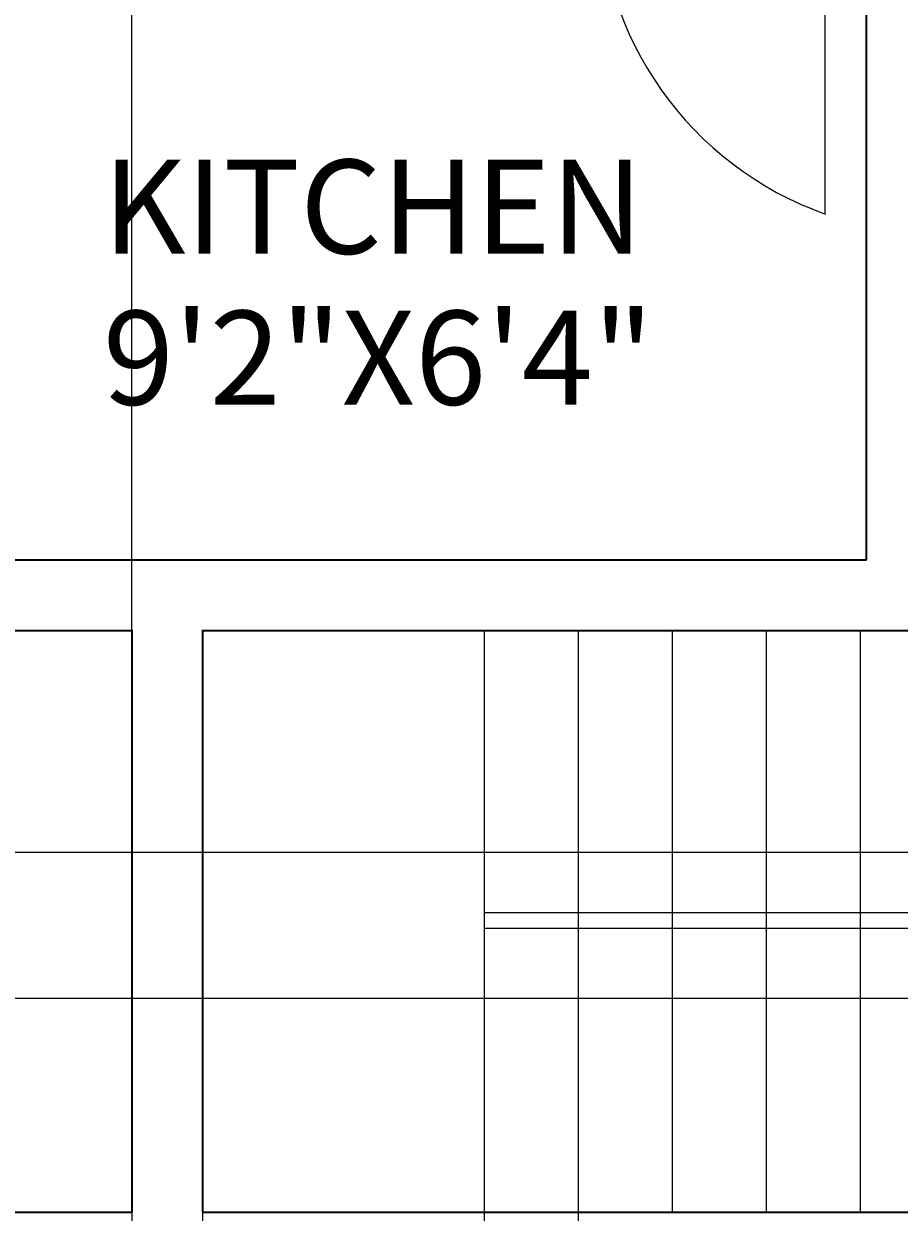
# Model space of a CAD drawing. Units: feet. Extents: x 5816 to 6644, y 25475 to 26788.
# Tile 4 of 23: x 5940 to 6052, y 26094 to 26246. Entities that reach past the tile are written whole.
import ezdxf

# ---------------------------------------------------------------- set-up
doc = ezdxf.new("R2010")
doc.units = ezdxf.units.FT
for name, color, linetype, lineweight in [('A-ANNO-DIMS', 2, 'Continuous', 13), ('A-AREA-IDEN', 7, 'Continuous', 18), ('A-DOOR', 3, 'Continuous', 18), ('A-FLOR-STRS', 7, 'Continuous', 18), ('A-WALL', 7, 'Continuous', 35)]:
    doc.layers.add(name, color=color, linetype=linetype, lineweight=lineweight)
doc.styles.get("Standard").update_dxf_attribs({"font": 'arial.ttf'})
doc.dimstyles.get("Standard").update_dxf_attribs({"dimtxt": 0.18, "dimasz": 0.18, "dimexe": 0.18, "dimexo": 0.0625, "dimgap": 0.09, "dimtad": 0, "dimtih": 1, "dimtoh": 1, "dimdec": 4, "dimzin": 0, "dimdsep": 46, "dimtxsty": 'Standard', "dimcen": 0.09, "dimadec": 0, "dimazin": 0, "dimtfac": 1, "dimtdec": 4, "dimtofl": 0, "dimtmove": 0, "dimatfit": 3, "dimfxl": 1, "dimtolj": 1, "dimtzin": 0, "dimarcsym": 0})

# ---------------------------------------------------------------- blocks, each defined once
blk = doc.blocks.new('DOOR-KITCHEN')
blk.add_line((0, -40.87), (0, 0))
blk.add_arc((14.45, 0), 43.35, 180, 250.5286)
blk = doc.blocks.new('*D58')
at = {"layer": 'A-ANNO-DIMS', "color": 0, "lineweight": -2, "transparency": 16777216}
for p, q in [((5953.98, 26168.65), (5953.98, 26787.91)), ((5954.16, 26787.73), (6030.2, 26787.73)), ((6106.8, 26787.73), (6030.76, 26787.73)), ((6106.98, 26168.71), (6106.98, 26787.91))]:
    blk.add_line(p, q, dxfattribs=at)
at = {"layer": 'A-ANNO-DIMS', "color": 0, "transparency": 16777216}
for points in [[(5954.16, 26787.76), (5954.16, 26787.7), (5953.98, 26787.73)], [(6106.8, 26787.76), (6106.8, 26787.7), (6106.98, 26787.73)]]:
    blk.add_solid(points, dxfattribs=at)
at = {"layer": 'Defpoints', "color": 0, "transparency": 16777216}
for p in [(6106.98, 26787.73), (5953.98, 26168.58), (6106.98, 26168.65)]:
    blk.add_point(p, dxfattribs=at)
at = {"layer": 'A-ANNO-DIMS', "color": 0, "transparency": 16777216, "insert": (6030.48, 26787.73), "char_height": 0.18, "attachment_point": 5}
blk.add_mtext('\\A1;153', dxfattribs=at)
blk = doc.blocks.new('*D62')
at = {"layer": 'A-ANNO-DIMS', "color": 0, "lineweight": -2, "transparency": 16777216}
for p, q in [((5877.31, 26168.52), (5877.31, 25475.01)), ((5953.98, 26168.52), (5953.98, 25475.01)), ((5877.49, 25475.19), (5915.25, 25475.19)), ((5953.8, 25475.19), (5916.04, 25475.19))]:
    blk.add_line(p, q, dxfattribs=at)
at = {"layer": 'A-ANNO-DIMS', "color": 0, "transparency": 16777216}
for points in [[(5877.49, 25475.22), (5877.49, 25475.16), (5877.31, 25475.19)], [(5953.8, 25475.22), (5953.8, 25475.16), (5953.98, 25475.19)]]:
    blk.add_solid(points, dxfattribs=at)
at = {"layer": 'Defpoints', "color": 0, "transparency": 16777216}
for p in [(5877.31, 26168.58), (5953.98, 26168.58), (5953.98, 25475.19)]:
    blk.add_point(p, dxfattribs=at)
at = {"layer": 'A-ANNO-DIMS', "color": 0, "transparency": 16777216, "insert": (5915.64, 25475.19), "char_height": 0.18, "attachment_point": 5}
blk.add_mtext('\\A1;76.67', dxfattribs=at)
blk = doc.blocks.new('*D67')
at = {"layer": 'A-ANNO-DIMS', "color": 0, "lineweight": -2, "transparency": 16777216}
for p, q in [((5998.98, 26094.27), (5998.98, 25475.01)), ((6010.98, 26094.27), (6010.98, 25475.01)), ((5999.16, 25475.19), (6004.77, 25475.19)), ((6010.8, 25475.19), (6005.19, 25475.19))]:
    blk.add_line(p, q, dxfattribs=at)
at = {"layer": 'A-ANNO-DIMS', "color": 0, "transparency": 16777216}
for points in [[(5999.16, 25475.22), (5999.16, 25475.16), (5998.98, 25475.19)], [(6010.8, 25475.22), (6010.8, 25475.16), (6010.98, 25475.19)]]:
    blk.add_solid(points, dxfattribs=at)
at = {"layer": 'Defpoints', "color": 0, "transparency": 16777216}
for p in [(5998.98, 26094.34), (6010.98, 26094.34), (6010.98, 25475.19)]:
    blk.add_point(p, dxfattribs=at)
at = {"layer": 'A-ANNO-DIMS', "color": 0, "transparency": 16777216, "insert": (6004.98, 25475.19), "char_height": 0.18, "attachment_point": 5}
blk.add_mtext('\\A1;12', dxfattribs=at)
blk = doc.blocks.new('*D68')
at = {"layer": 'A-ANNO-DIMS', "color": 0, "lineweight": -2, "transparency": 16777216}
for p, q in [((5962.98, 26094.27), (5962.98, 25475.01)), ((5998.98, 26094.27), (5998.98, 25475.01)), ((5963.16, 25475.19), (5980.76, 25475.19)), ((5998.8, 25475.19), (5981.2, 25475.19))]:
    blk.add_line(p, q, dxfattribs=at)
at = {"layer": 'A-ANNO-DIMS', "color": 0, "transparency": 16777216}
for points in [[(5963.16, 25475.22), (5963.16, 25475.16), (5962.98, 25475.19)], [(5998.8, 25475.22), (5998.8, 25475.16), (5998.98, 25475.19)]]:
    blk.add_solid(points, dxfattribs=at)
at = {"layer": 'Defpoints', "color": 0, "transparency": 16777216}
for p in [(5962.98, 26094.34), (5998.98, 26094.34), (5998.98, 25475.19)]:
    blk.add_point(p, dxfattribs=at)
at = {"layer": 'A-ANNO-DIMS', "color": 0, "transparency": 16777216, "insert": (5980.98, 25475.19), "char_height": 0.18, "attachment_point": 5}
blk.add_mtext('\\A1;36', dxfattribs=at)
blk = doc.blocks.new('*D71')
at = {"layer": 'A-ANNO-DIMS', "color": 0, "lineweight": -2, "transparency": 16777216}
for p, q in [((6343.61, 26140.22), (5815.98, 26140.22)), ((5816.16, 26140.04), (5816.16, 26131.1)), ((5816.16, 26121.79), (5816.16, 26130.74)), ((6343.61, 26121.61), (5815.98, 26121.61))]:
    blk.add_line(p, q, dxfattribs=at)
at = {"layer": 'A-ANNO-DIMS', "color": 0, "transparency": 16777216}
for points in [[(5816.13, 26140.04), (5816.19, 26140.04), (5816.16, 26140.22)], [(5816.13, 26121.79), (5816.19, 26121.79), (5816.16, 26121.61)]]:
    blk.add_solid(points, dxfattribs=at)
at = {"layer": 'Defpoints', "color": 0, "transparency": 16777216}
for p in [(6343.68, 26140.22), (5816.16, 26121.61), (6343.68, 26121.61)]:
    blk.add_point(p, dxfattribs=at)
at = {"layer": 'A-ANNO-DIMS', "color": 0, "transparency": 16777216, "insert": (5816.16, 26130.92), "char_height": 0.18, "attachment_point": 5}
blk.add_mtext('\\A1;18.61', dxfattribs=at)

msp = doc.modelspace()

# ---------------------------------------------------------------- linework, layer by layer
at = {"layer": 'A-FLOR-STRS'}
for p, q in [((5998.9781, 26168.6509), (5998.9781, 26094.3368)), ((6010.9781, 26168.6509), (6010.9781, 26094.3368)), ((6022.9781, 26168.6509), (6022.9781, 26094.3368)), ((6034.9781, 26168.6509), (6034.9781, 26094.3368)), ((6046.9781, 26168.6509), (6046.9781, 26094.3368)), ((5998.9781, 26132.5846), (6106.9781, 26132.5846)), ((5998.9781, 26130.5846), (6106.9781, 26130.5846))]:
    msp.add_line(p, q, dxfattribs=at)
at = {"layer": 'A-WALL'}
for p, q in [((6047.8119, 26177.5846), (6047.8119, 26262.5846)), ((5933.3119, 26177.5846), (6047.8119, 26177.5846)), ((5877.3119, 26168.5846), (5953.9781, 26168.5846)), ((5953.9781, 26168.6509), (5953.9781, 26094.3368)), ((5962.9781, 26168.6509), (5962.9781, 26094.3368)), ((5962.9781, 26168.5846), (6175.0829, 26168.5846)), ((5933.3119, 26094.3368), (5953.9781, 26094.3368)), ((5962.9781, 26094.3368), (6175.0829, 26094.3368))]:
    msp.add_line(p, q, dxfattribs=at)

# ---------------------------------------------------------------- block references
at = {"layer": 'A-DOOR'}
msp.add_blockref('DOOR-KITCHEN', (6042.532, 26262.5846), dxfattribs=at)

# ---------------------------------------------------------------- texts
at = {"layer": 'A-ANNO-DIMS'}
msp.add_text('9\'2"X6\'4"', height=12, dxfattribs=at).set_placement((5950.2747, 26197.3709))
at = {"layer": 'A-AREA-IDEN'}
msp.add_text('KITCHEN', height=12, dxfattribs=at).set_placement((5950.2747, 26216.6479))

# ---------------------------------------------------------------- dimensions: what is measured, and where the dimension line sits
at = {"layer": 'A-ANNO-DIMS'}
for base, p1, p2, override, picture, middle in [((6106.9781, 26787.7346), (5953.9781, 26168.5846), (6106.9781, 26168.6509), {"dimdec": 0, "dimlfac": 1, "dimrnd": 0, "dimzin": 0, "dimdsep": 46, "dimlunit": 2}, '*D58', (6030.4781, 26787.7346)), ((5953.9781, 25475.1868), (5877.3119, 26168.5846), (5953.9781, 26168.5846), {"dimdec": 2, "dimlfac": 1, "dimrnd": 0, "dimzin": 0, "dimdsep": 46, "dimlunit": 2}, '*D62', (5915.645, 25475.1868)), ((5998.9781, 25475.1868), (5962.9781, 26094.3368), (5998.9781, 26094.3368), {"dimdec": 0, "dimlfac": 1, "dimrnd": 0, "dimzin": 0, "dimdsep": 46, "dimlunit": 2}, '*D68', (5980.9781, 25475.1868)), ((6010.9781, 25475.1868), (5998.9781, 26094.3368), (6010.9781, 26094.3368), {"dimdec": 0, "dimlfac": 1, "dimrnd": 0, "dimzin": 0, "dimdsep": 46, "dimlunit": 2}, '*D67', (6004.9781, 25475.1868))]:
    dim = msp.add_linear_dim(base=base, p1=p1, p2=p2, dimstyle='Standard', override=override, dxfattribs=at)
    dim.commit()
    dim.dimension.update_dxf_attribs({"geometry": picture, "text_midpoint": middle})
dim = msp.add_linear_dim(base=(5816.1619, 26121.6124), p1=(6343.6763, 26140.2241), p2=(6343.6763, 26121.6124), angle=90, dimstyle='Standard', override={"dimdec": 2, "dimlfac": 1, "dimrnd": 0, "dimzin": 0, "dimdsep": 46, "dimlunit": 2}, dxfattribs=at)
dim.commit()
dim.dimension.update_dxf_attribs({"geometry": '*D71', "text_midpoint": (5816.1619, 26130.9183)})

doc.saveas('drawing.dxf')
